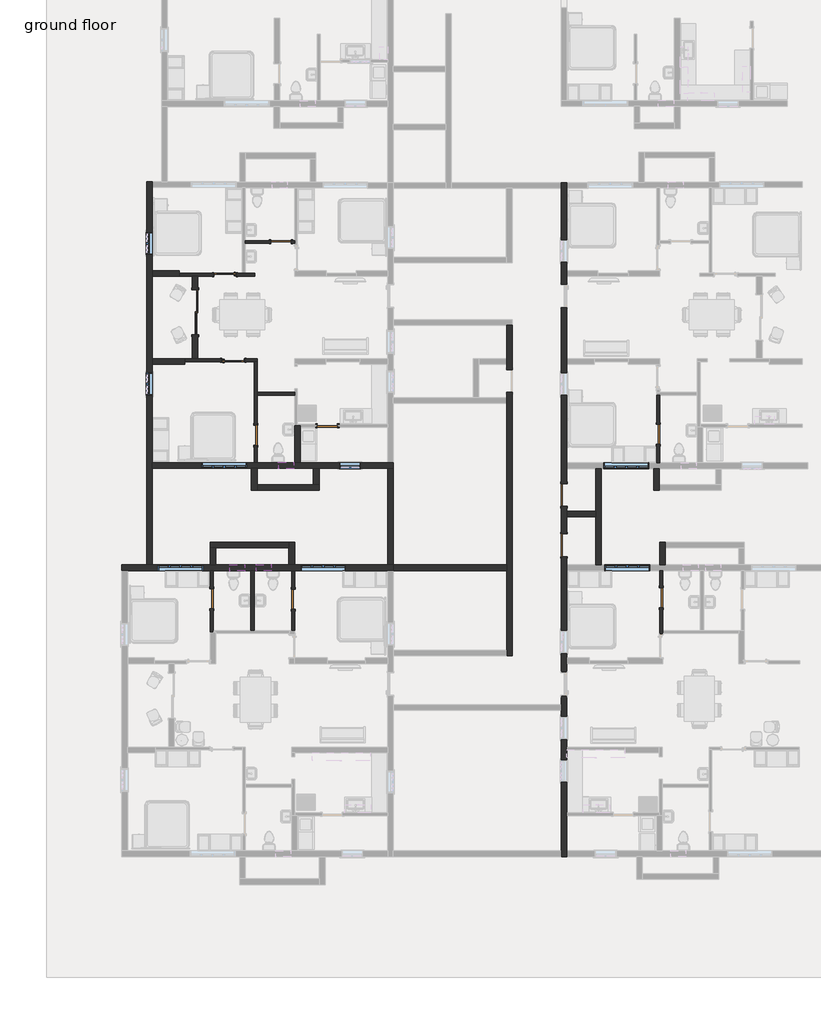
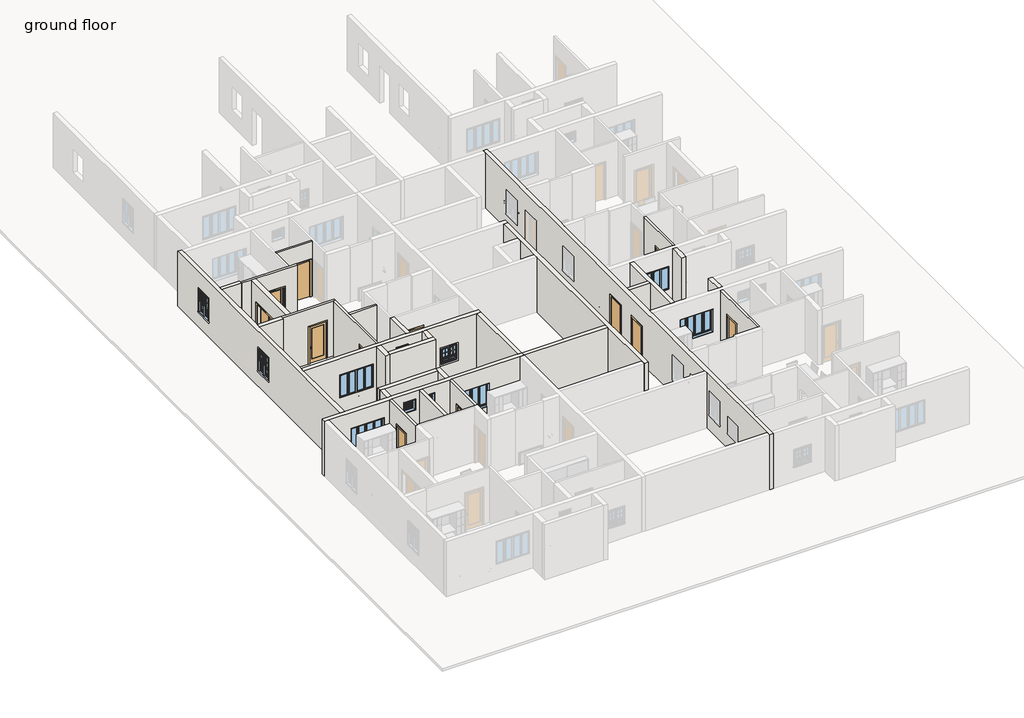
# One storey, part 2 of 16: 31 walls, 12 doors, 11 windows.
# Revit data of these elements (continued)
# Element 22 (IfcWall, "Generic - 6\"") (continued)
#   Base Offset = 0' - 0"
#   wall height = 10' - 6"
#   Phase Created = New Construction
#   Base Constraint = ground floor
#   Top Constraint = 1st floor
#   Materials on its faces: "Default Wall"
# Elements 23, 24, 25, 26, 27, 28, 29, 30, 31, 32, 33, 34, 35, 36, 37, 38, 39, 40, 41, 42, 43 (IfcWall, "Generic - 9\"")
#   Top Offset = 0' - 0"
#   Base Offset = 0' - 0"
#   wall height = 10' - 6"
#   Phase Created = New Construction
#   Base Constraint = ground floor
#   Top Constraint = 1st floor
#   Materials on its faces: "Default Wall"
# Element 44 (IfcWindow, "Window-Casement-Double-Awning : 34\" x 36\"")
#   Mark = "83"
#   Window Inset = 0' - 0"
#   Interior Wall Closure = 0' - 2 1/4"
#   Frame Extension = 0' - 0 1/4"
#   Exterior Wall Closure = 0' - 1 1/4"
#   Interior Trim Visibility = yes
#   Exterior Trim Visibility = yes
#   Phase Created = New Construction
#   Materials on its faces: "Wood - Stained", "Glass", "Clad - White"
# Element 45 (IfcWindow, "Window-Casement-Multi-Sash-Horizontal : 72\" x 53\"")
#   Mark = "28"
#   Window Inset = 0' - 0 5/8"
#   Frame Gap 3 = 0' - 1 83/128"
#   Frame Gap 2 = 0' - 0 5/8"
#   Phase Created = New Construction
#   Materials on its faces: "Metal - Aluminum", "Glass"
# Element 46 (IfcWindow, "Window-Casement-Multi-Sash-Horizontal : 72\" x 53\"")
#   Mark = "29"
#   Window Inset = 0' - 0 5/8"
#   Frame Gap 3 = 0' - 1 83/128"
#   Frame Gap 2 = 0' - 0 5/8"
#   Phase Created = New Construction
#   Materials on its faces: "Metal - Aluminum", "Glass"
# Element 47 (IfcWindow, "Window-Casement-Multi-Sash-Horizontal : 72\" x 53\"")
#   Mark = "32"
#   Window Inset = 0' - 0 5/8"
#   Frame Gap 3 = 0' - 1 83/128"
#   Frame Gap 2 = 0' - 0 5/8"
#   Phase Created = New Construction
#   Materials on its faces: "Metal - Aluminum", "Glass"
# Element 48 (IfcWindow, "Window-Casement-Multi-Sash-Horizontal : 72\" x 53\"")
#   Mark = "33"
#   Window Inset = 0' - 0 5/8"
#   Frame Gap 3 = 0' - 1 83/128"
#   Frame Gap 2 = 0' - 0 5/8"
#   Phase Created = New Construction
#   Materials on its faces: "Metal - Aluminum", "Glass"
# Element 49 (IfcWindow, "Window-Casement-Multi-Sash-Horizontal : 72\" x 53\"")
#   Mark = "34"
#   Window Inset = 0' - 0 5/8"
#   Frame Gap 3 = 0' - 1 83/128"
#   Frame Gap 2 = 0' - 0 5/8"
#   Phase Created = New Construction
#   Materials on its faces: "Metal - Aluminum", "Glass"
# Element 50 (IfcWindow, "Window-Louvers : 24\" x 24\"")
#   Mark = "104"
#   Blade Width = 1' - 10 1/2"
#   Phase Created = New Construction
#   Materials on its faces: "Birch"
# Element 51 (IfcWindow, "Window-Louvers : 24\" x 24\"")
#   Mark = "105"
#   Blade Width = 1' - 10 1/2"
#   Phase Created = New Construction
#   Materials on its faces: "Birch"
# Element 52 (IfcWindow, "Window-Louvers : 24\" x 24\"")
#   Mark = "106"
#   Blade Width = 1' - 10 1/2"
#   Phase Created = New Construction
#   Materials on its faces: "Birch"
# Element 53 (IfcWindow, "Window-Single-Hung-Double : 36\" x 52\"")
#   Mark = "58"
#   Window Inset = 0' - 0"
#   Interior Wall Closure = 0' - 1 1/2"
#   Frame Extension = 0' - 1 1/4"
#   Exterior Wall Closure = 0' - 0 1/2"
#   Interior Trim Visibility = yes
#   Indicator Visibility = yes
#   Exterior Trim Visibility = yes
#   Phase Created = New Construction
#   Materials on its faces: "Wood - Stained", "Glass", "Clad - White"
# Element 54 (IfcWindow, "Window-Single-Hung-Double : 36\" x 52\"")
#   Mark = "59"
#   Window Inset = 0' - 0"
#   Interior Wall Closure = 0' - 1 1/2"
#   Frame Extension = 0' - 1 1/4"
#   Exterior Wall Closure = 0' - 0 1/2"
#   Interior Trim Visibility = yes
#   Indicator Visibility = yes
#   Exterior Trim Visibility = yes
#   Phase Created = New Construction
#   Materials on its faces: "Wood - Stained", "Glass", "Clad - White"
# Materials
#   "Glass": class "Glass", colour RGB 0 128 192, transparency 0.75, Description = "Soda Lime Glass", Cost = 0
#   "Wood - Birch - Solid Stained Light Low Gloss": class "Wood", colour RGB 210 159 95, transparency 0, Cost = 0
#   "Paint - Sienna": colour RGB 118 70 51, transparency 0, Cost = 0
#   "Cherry": class "Wood", colour RGB 226 177 128, transparency 0, Description = "Prunus Serotina", Cost = 0
#   "Aluminum": class "Metal", colour RGB 247 247 247, transparency 0, Description = "Aluminum 6061", Cost = 0
#   "Door - Panel": class "Wood", colour RGB 210 159 95, transparency 0, Cost = 0
#   "Door - Frame": colour RGB 118 70 51, transparency 0, Cost = 0
#   "Wood - Stained": class "Wood", colour RGB 224 178 126, transparency 0, Cost = 0
#   "Clad - White": class "Wood", colour RGB 242 242 238, transparency 0, Cost = 0
#   "Metal - Aluminum": class "Metal", colour RGB 247 247 247, transparency 0
#   "Birch": class "Wood", colour RGB 224 178 126, transparency 0, Description = "Betula Alleghaniensis", Cost = 0
#   "Default Wall": colour RGB 128 128 128, transparency 0, Cost = 0
